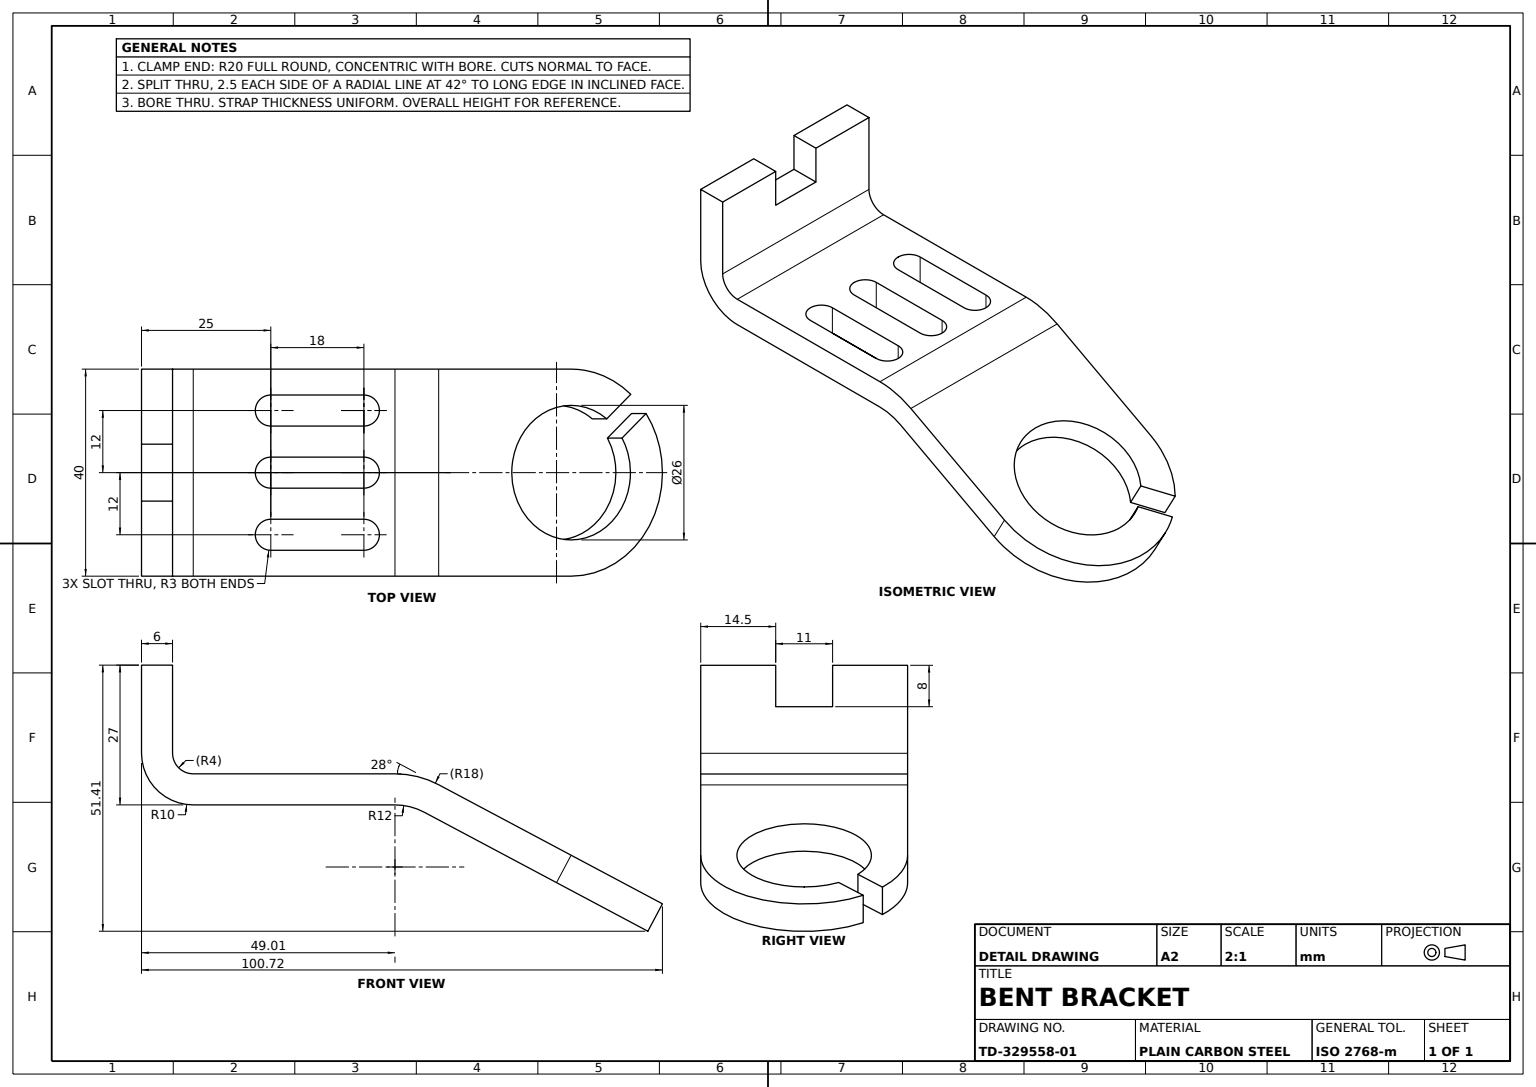
from build123d import *

# Parameters (mm, degrees)
BENT_STRAP_BODY_DEPTH      = 40
SLOTS_3X6_WIDE_REACH       = 118.826
SPLIT_CLAMP_RING_CUT_REACH = 114.485
END_TAB_NOTCH_11X8_REACH   = 108.308
END_TAB_NOTCH_SKETCH_W     = 11
END_TAB_NOTCH_SKETCH_H     = 16


with BuildPart() as part:
    # Strap Profile Sketch → Bent Strap Body (new body)
    with BuildSketch(Plane.XY):
        with BuildLine():
            Line((0, 27), (0, 10))
            ThreePointArc((0, 10), (2.928932188, 2.928932188), (10, 0))
            Line((10, 0), (49.008063966, 0))
            ThreePointArc((49.008063966, 0), (51.911126713, -0.356451285), (54.641722719, -1.404628886))
            Line((54.641722719, -1.404628886), (102, -26.585471583))
            Line((102, -26.585471583), (104.816829377, -21.287786026))
            Line((104.816829377, -21.287786026), (57.458552096, 3.893056671))
            ThreePointArc((57.458552096, 3.893056671), (53.362658087, 5.465323073), (49.008063966, 6))
            Line((49.008063966, 6), (10, 6))
            ThreePointArc((10, 6), (7.171572875, 7.171572875), (6, 10))
            Line((6, 10), (6, 27))
            Line((6, 27), (0, 27))
        make_face()
    extrude(amount=BENT_STRAP_BODY_DEPTH)

    # Slots Sketch → Slots 3x6 Wide (cut, up to next)
    with BuildSketch(Plane(origin=(0, 6, 0), x_dir=(1, 0, 0), z_dir=(0, 1, 0)), mode=Mode.PRIVATE) as slots_3x6_wide_sk1:
        with BuildLine():
            Line((25, -17), (43, -17))
            ThreePointArc((43, -17), (46, -20), (43, -23))
            Line((43, -23), (25, -23))
            ThreePointArc((25, -23), (22, -20), (25, -17))
        make_face()
    slots_3x6_wide_tool1 = extrude(slots_3x6_wide_sk1.sketch, amount=-SLOTS_3X6_WIDE_REACH, mode=Mode.PRIVATE) & part.part
    # Slots Sketch → Slots 3x6 Wide (cut, up to next)
    with BuildSketch(Plane(origin=(0, 6, 0), x_dir=(1, 0, 0), z_dir=(0, 1, 0)), mode=Mode.PRIVATE) as slots_3x6_wide_sk2:
        with BuildLine():
            Line((25, -5), (43, -5))
            ThreePointArc((43, -5), (46, -8), (43, -11))
            Line((43, -11), (25, -11))
            ThreePointArc((25, -11), (22, -8), (25, -5))
        make_face()
    slots_3x6_wide_tool2 = extrude(slots_3x6_wide_sk2.sketch, amount=-SLOTS_3X6_WIDE_REACH, mode=Mode.PRIVATE) & part.part
    # Slots Sketch → Slots 3x6 Wide (cut, up to next)
    with BuildSketch(Plane(origin=(0, 6, 0), x_dir=(1, 0, 0), z_dir=(0, 1, 0)), mode=Mode.PRIVATE) as slots_3x6_wide_sk3:
        with BuildLine():
            Line((25, -29), (43, -29))
            ThreePointArc((43, -29), (46, -32), (43, -35))
            Line((43, -35), (25, -35))
            ThreePointArc((25, -35), (22, -32), (25, -29))
        make_face()
    slots_3x6_wide_tool3 = extrude(slots_3x6_wide_sk3.sketch, amount=-SLOTS_3X6_WIDE_REACH, mode=Mode.PRIVATE) & part.part
    add(slots_3x6_wide_tool1.solids().sort_by_distance((34, 6, 20))[0], mode=Mode.SUBTRACT)
    add(slots_3x6_wide_tool2.solids().sort_by_distance((34, 6, 8))[0], mode=Mode.SUBTRACT)
    add(slots_3x6_wide_tool3.solids().sort_by_distance((34, 6, 32))[0], mode=Mode.SUBTRACT)

    # Split Clamp Ring Sketch → Split Clamp Ring Cut (cut, up to next)
    with BuildSketch(Plane(origin=(14.277813886, 26.852662444, 0), x_dir=(0.8829475928589264, -0.46947156278589186, 0), z_dir=(0.46947156278589186, 0.8829475928589264, 0)), mode=Mode.PRIVATE) as split_clamp_ring_cut_sk1:
        with BuildLine():
            Line((90.978707319, -4.864489093), (85.712943597, -9.605804045))
            ThreePointArc((85.712943597, -9.605804045), (68.244328132, -28.698697883), (89.058596629, -13.321528173))
            Line((89.058596629, -13.321528173), (94.324360351, -8.580213221))
            ThreePointArc((94.324360351, -8.580213221), (95.630838293, -29.262944036), (77.905210863, -40))
            Line((77.905210863, -40), (102.541777363, -40))
            Line((102.541777363, -40), (102.541777363, 0))
            Line((102.541777363, 0), (77.905210863, 0))
            ThreePointArc((77.905210863, 0), (84.879799807, -1.255531241), (90.978707319, -4.864489093))
        make_face()
    split_clamp_ring_cut_tool1 = extrude(split_clamp_ring_cut_sk1.sketch, amount=-SPLIT_CLAMP_RING_CUT_REACH, mode=Mode.PRIVATE) & part.part
    add(split_clamp_ring_cut_tool1.solids().sort_by_distance((89.983505, -13.400768, 19.581438))[0], mode=Mode.SUBTRACT)

    # End Tab Notch Sketch → End Tab Notch 11x8 (cut, up to next)
    with BuildSketch(Plane(origin=(6, 0, 0), x_dir=(0, 0, -1), z_dir=(1, 0, 0)), mode=Mode.PRIVATE) as end_tab_notch_11x8_sk1:
        with Locations((-20, 27)):
            Rectangle(END_TAB_NOTCH_SKETCH_W, END_TAB_NOTCH_SKETCH_H)
    end_tab_notch_11x8_tool1 = extrude(end_tab_notch_11x8_sk1.sketch, amount=-END_TAB_NOTCH_11X8_REACH, mode=Mode.PRIVATE) & part.part
    add(end_tab_notch_11x8_tool1.solids().sort_by_distance((6, 27, 20))[0], mode=Mode.SUBTRACT)


solid = part.part
